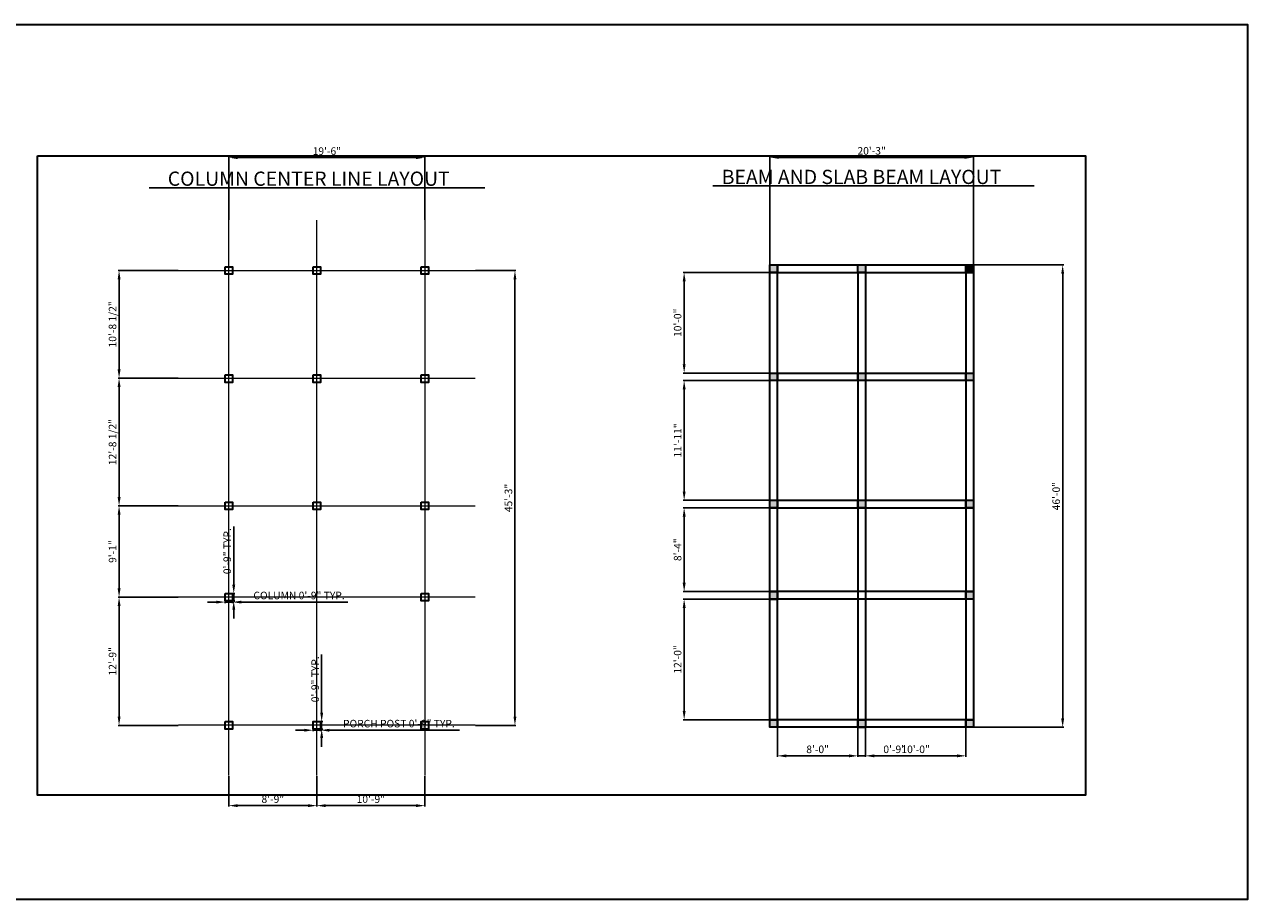
# Model space of a CAD drawing. Units: inches. Extents: x 1956 to 4770, y 1551 to 2596.
# Tile 10 of 10: x 3310 to 4770, y 1551 to 2596. Entities that reach past the tile are written whole.
import ezdxf

# ---------------------------------------------------------------- set-up
doc = ezdxf.new("R2010")
doc.units = ezdxf.units.IN
doc.linetypes.add('ACAD_ISO02W100', pattern=[15, 12, -3])
for name, color, linetype, lineweight in [('A-ANNO-DIMS', 2, 'Continuous', 18), ('A-ANNO-TITL', 6, 'Continuous', 25), ('A-ANNO-TTLB', 7, 'Continuous', 35), ('S-BEAM', 7, 'Continuous', 35), ('S-COLS', 5, 'Continuous', 35), ('S-COLS-HIDN', 5, 'ACAD_ISO02W100', 18), ('S-COLS-PATT', 1, 'Continuous', 13), ('S-GRID', 1, 'Continuous', 13)]:
    doc.layers.add(name, color=color, linetype=linetype, lineweight=lineweight)
doc.styles.get("Standard").update_dxf_attribs({"font": 'arial.ttf'})
doc.dimstyles.new('ISO-25', dxfattribs={"dimtxt": 9, "dimasz": 10.5, "dimexe": 1.25, "dimexo": 0.625, "dimgap": 2, "dimtad": 1, "dimdec": 1, "dimlunit": 4, "dimtxsty": 'Standard', "dimcen": 2.5, "dimadec": 0, "dimazin": 0, "dimtfac": 1, "dimtdec": 1, "dimtmove": 0, "dimatfit": 3, "dimfxl": 1, "dimarcsym": 0})

# ---------------------------------------------------------------- blocks, each defined once
blk = doc.blocks.new('COL-9X9-PLAN')
blk.add_lwpolyline([(0, 9), (9, 9), (9, 0), (0, 0)], close=True)
blk = doc.blocks.new('COL-PORCH-9X9')
blk.add_line((0, 0), (9, 0))
blk.add_lwpolyline([(0, 0), (0, 9), (9, 9), (9, 0)])
blk = doc.blocks.new('*D23')
at = {"layer": 'A-ANNO-DIMS', "color": 0, "lineweight": -2, "transparency": 16777216}
for p, q in [((3538.6, 1906.6), (3528.1, 1906.6)), ((3549.1, 1907.3), (3549.1, 1905.3)), ((3549.1, 1906.6), (3558.1, 1906.6)), ((3558.1, 1907.3), (3558.1, 1905.3)), ((3568.6, 1906.6), (3695.8, 1906.6))]:
    blk.add_line(p, q, dxfattribs=at)
at = {"layer": 'A-ANNO-DIMS', "color": 0, "transparency": 16777216}
for points in [[(3538.6, 1908.3), (3538.6, 1904.8), (3549.1, 1906.6)], [(3568.6, 1908.3), (3568.6, 1904.8), (3558.1, 1906.6)]]:
    blk.add_solid(points, dxfattribs=at)
at = {"layer": 'Defpoints', "color": 0, "transparency": 16777216}
for p in [(3549.1, 1907.9), (3558.1, 1907.9), (3558.1, 1906.6)]:
    blk.add_point(p, dxfattribs=at)
at = {"layer": 'A-ANNO-DIMS', "color": 0, "transparency": 16777216, "insert": (3637.4, 1913.3), "char_height": 9, "attachment_point": 5}
blk.add_mtext('COLUMN 0\'-9" TYP.', dxfattribs=at)
blk = doc.blocks.new('*D24')
at = {"layer": 'A-ANNO-DIMS', "color": 0, "lineweight": -2, "transparency": 16777216}
for p, q in [((3559.4, 1927.4), (3559.4, 1996.8)), ((3558.7, 1916.9), (3560.7, 1916.9)), ((3559.4, 1907.9), (3559.4, 1916.9)), ((3558.7, 1907.9), (3560.7, 1907.9)), ((3559.4, 1897.4), (3559.4, 1886.9))]:
    blk.add_line(p, q, dxfattribs=at)
at = {"layer": 'A-ANNO-DIMS', "color": 0, "transparency": 16777216}
for points in [[(3557.7, 1927.4), (3561.2, 1927.4), (3559.4, 1916.9)], [(3557.7, 1897.4), (3561.2, 1897.4), (3559.4, 1907.9)]]:
    blk.add_solid(points, dxfattribs=at)
at = {"layer": 'Defpoints', "color": 0, "transparency": 16777216}
for p in [(3558.1, 1916.9), (3559.4, 1916.9), (3558.1, 1907.9)]:
    blk.add_point(p, dxfattribs=at)
at = {"layer": 'A-ANNO-DIMS', "color": 0, "transparency": 16777216, "insert": (3552.8, 1967.4), "char_height": 9, "attachment_point": 5, "rotation": 90}
blk.add_mtext('0\'-9" TYP.', dxfattribs=at)
blk = doc.blocks.new('*D25')
at = {"layer": 'A-ANNO-DIMS', "color": 0, "lineweight": -2, "transparency": 16777216}
for p, q in [((3643.6, 1753.6), (3633.1, 1753.6)), ((3654.1, 1754.3), (3654.1, 1752.3)), ((3654.1, 1753.6), (3663.1, 1753.6)), ((3663.1, 1754.3), (3663.1, 1752.3)), ((3673.6, 1753.6), (3829.1, 1753.6))]:
    blk.add_line(p, q, dxfattribs=at)
at = {"layer": 'A-ANNO-DIMS', "color": 0, "transparency": 16777216}
for points in [[(3643.6, 1755.3), (3643.6, 1751.8), (3654.1, 1753.6)], [(3673.6, 1755.3), (3673.6, 1751.8), (3663.1, 1753.6)]]:
    blk.add_solid(points, dxfattribs=at)
at = {"layer": 'Defpoints', "color": 0, "transparency": 16777216}
for p in [(3654.1, 1754.9), (3663.1, 1754.9), (3663.1, 1753.6)]:
    blk.add_point(p, dxfattribs=at)
at = {"layer": 'A-ANNO-DIMS', "color": 0, "transparency": 16777216, "insert": (3756.6, 1760.3), "char_height": 9, "attachment_point": 5}
blk.add_mtext('PORCH POST 0\'-9" TYP.', dxfattribs=at)
blk = doc.blocks.new('*D26')
at = {"layer": 'A-ANNO-DIMS', "color": 0, "lineweight": -2, "transparency": 16777216}
for p, q in [((3664.4, 1774.4), (3664.4, 1843.8)), ((3663.7, 1763.9), (3665.7, 1763.9)), ((3663.7, 1754.9), (3665.7, 1754.9)), ((3664.4, 1754.9), (3664.4, 1763.9)), ((3664.4, 1744.4), (3664.4, 1733.9))]:
    blk.add_line(p, q, dxfattribs=at)
at = {"layer": 'A-ANNO-DIMS', "color": 0, "transparency": 16777216}
for points in [[(3662.7, 1774.4), (3666.2, 1774.4), (3664.4, 1763.9)], [(3662.7, 1744.4), (3666.2, 1744.4), (3664.4, 1754.9)]]:
    blk.add_solid(points, dxfattribs=at)
at = {"layer": 'Defpoints', "color": 0, "transparency": 16777216}
for p in [(3663.1, 1763.9), (3663.1, 1754.9), (3664.4, 1763.9)]:
    blk.add_point(p, dxfattribs=at)
at = {"layer": 'A-ANNO-DIMS', "color": 0, "transparency": 16777216, "insert": (3657.8, 1814.4), "char_height": 9, "attachment_point": 5, "rotation": 90}
blk.add_mtext('0\'-9" TYP.', dxfattribs=at)
blk = doc.blocks.new('*D87')
at = {"layer": 'A-ANNO-DIMS', "color": 0, "lineweight": -2, "transparency": 16777216}
for p, q in [((3553.6, 1698.8), (3553.6, 1662.3)), ((3658.6, 1698.8), (3658.6, 1662.3)), ((3564.1, 1663.5), (3648.1, 1663.5))]:
    blk.add_line(p, q, dxfattribs=at)
at = {"layer": 'A-ANNO-DIMS', "color": 0, "transparency": 16777216}
for points in [[(3564.1, 1665.3), (3564.1, 1661.8), (3553.6, 1663.5)], [(3648.1, 1665.3), (3648.1, 1661.8), (3658.6, 1663.5)]]:
    blk.add_solid(points, dxfattribs=at)
at = {"layer": 'Defpoints', "color": 0, "transparency": 16777216}
for p in [(3553.6, 1699.4), (3658.6, 1699.4), (3658.6, 1663.5)]:
    blk.add_point(p, dxfattribs=at)
at = {"layer": 'A-ANNO-DIMS', "color": 0, "transparency": 16777216, "insert": (3606.1, 1670.1), "char_height": 9, "attachment_point": 5}
blk.add_mtext('8\'-9"', dxfattribs=at)
blk = doc.blocks.new('*D88')
at = {"layer": 'A-ANNO-DIMS', "color": 0, "lineweight": -2, "transparency": 16777216}
for p, q in [((3658.6, 1698.8), (3658.6, 1662.3)), ((3787.6, 1698.8), (3787.6, 1662.3)), ((3669.1, 1663.5), (3777.1, 1663.5))]:
    blk.add_line(p, q, dxfattribs=at)
at = {"layer": 'A-ANNO-DIMS', "color": 0, "transparency": 16777216}
for points in [[(3669.1, 1665.3), (3669.1, 1661.8), (3658.6, 1663.5)], [(3777.1, 1665.3), (3777.1, 1661.8), (3787.6, 1663.5)]]:
    blk.add_solid(points, dxfattribs=at)
at = {"layer": 'Defpoints', "color": 0, "transparency": 16777216}
for p in [(3658.6, 1699.4), (3787.6, 1699.4), (3787.6, 1663.5)]:
    blk.add_point(p, dxfattribs=at)
at = {"layer": 'A-ANNO-DIMS', "color": 0, "transparency": 16777216, "insert": (3723.1, 1670.1), "char_height": 9, "attachment_point": 5}
blk.add_mtext('10\'-9"', dxfattribs=at)
blk = doc.blocks.new('*D89')
at = {"layer": 'A-ANNO-DIMS', "color": 0, "lineweight": -2, "transparency": 16777216}
for p, q in [((3492.9, 1912.4), (3421.3, 1912.4)), ((3422.5, 1769.9), (3422.5, 1901.9)), ((3492.9, 1759.4), (3421.3, 1759.4))]:
    blk.add_line(p, q, dxfattribs=at)
at = {"layer": 'A-ANNO-DIMS', "color": 0, "transparency": 16777216}
for points in [[(3420.8, 1901.9), (3424.3, 1901.9), (3422.5, 1912.4)], [(3420.8, 1769.9), (3424.3, 1769.9), (3422.5, 1759.4)]]:
    blk.add_solid(points, dxfattribs=at)
at = {"layer": 'Defpoints', "color": 0, "transparency": 16777216}
for p in [(3422.5, 1912.4), (3493.6, 1912.4), (3493.6, 1759.4)]:
    blk.add_point(p, dxfattribs=at)
at = {"layer": 'A-ANNO-DIMS', "color": 0, "transparency": 16777216, "insert": (3415.9, 1835.9), "char_height": 9, "attachment_point": 5, "rotation": 90}
blk.add_mtext('12\'-9"', dxfattribs=at)
blk = doc.blocks.new('*D90')
at = {"layer": 'A-ANNO-DIMS', "color": 0, "lineweight": -2, "transparency": 16777216}
for p, q in [((3492.9, 2021.4), (3421.3, 2021.4)), ((3422.5, 1922.9), (3422.5, 2010.9)), ((3492.9, 1912.4), (3421.3, 1912.4))]:
    blk.add_line(p, q, dxfattribs=at)
at = {"layer": 'A-ANNO-DIMS', "color": 0, "transparency": 16777216}
for points in [[(3420.8, 2010.9), (3424.3, 2010.9), (3422.5, 2021.4)], [(3420.8, 1922.9), (3424.3, 1922.9), (3422.5, 1912.4)]]:
    blk.add_solid(points, dxfattribs=at)
at = {"layer": 'Defpoints', "color": 0, "transparency": 16777216}
for p in [(3422.5, 2021.4), (3493.6, 2021.4), (3493.6, 1912.4)]:
    blk.add_point(p, dxfattribs=at)
at = {"layer": 'A-ANNO-DIMS', "color": 0, "transparency": 16777216, "insert": (3415.9, 1966.9), "char_height": 9, "attachment_point": 5, "rotation": 90}
blk.add_mtext('9\'-1"', dxfattribs=at)
blk = doc.blocks.new('*D91')
at = {"layer": 'A-ANNO-DIMS', "color": 0, "lineweight": -2, "transparency": 16777216}
for p, q in [((3492.9, 2173.9), (3421.3, 2173.9)), ((3422.5, 2031.9), (3422.5, 2163.4)), ((3492.9, 2021.4), (3421.3, 2021.4))]:
    blk.add_line(p, q, dxfattribs=at)
at = {"layer": 'A-ANNO-DIMS', "color": 0, "transparency": 16777216}
for points in [[(3420.8, 2163.4), (3424.3, 2163.4), (3422.5, 2173.9)], [(3420.8, 2031.9), (3424.3, 2031.9), (3422.5, 2021.4)]]:
    blk.add_solid(points, dxfattribs=at)
at = {"layer": 'Defpoints', "color": 0, "transparency": 16777216}
for p in [(3422.5, 2173.9), (3493.6, 2173.9), (3493.6, 2021.4)]:
    blk.add_point(p, dxfattribs=at)
at = {"layer": 'A-ANNO-DIMS', "color": 0, "transparency": 16777216, "insert": (3415.9, 2097.7), "char_height": 9, "attachment_point": 5, "rotation": 90}
blk.add_mtext('12\'-8 1/2"', dxfattribs=at)
blk = doc.blocks.new('*D92')
at = {"layer": 'A-ANNO-DIMS', "color": 0, "lineweight": -2, "transparency": 16777216}
for p, q in [((3492.9, 2302.4), (3421.3, 2302.4)), ((3422.5, 2184.4), (3422.5, 2291.9)), ((3492.9, 2173.9), (3421.3, 2173.9))]:
    blk.add_line(p, q, dxfattribs=at)
at = {"layer": 'A-ANNO-DIMS', "color": 0, "transparency": 16777216}
for points in [[(3420.8, 2291.9), (3424.3, 2291.9), (3422.5, 2302.4)], [(3420.8, 2184.4), (3424.3, 2184.4), (3422.5, 2173.9)]]:
    blk.add_solid(points, dxfattribs=at)
at = {"layer": 'Defpoints', "color": 0, "transparency": 16777216}
for p in [(3422.5, 2302.4), (3493.6, 2302.4), (3493.6, 2173.9)]:
    blk.add_point(p, dxfattribs=at)
at = {"layer": 'A-ANNO-DIMS', "color": 0, "transparency": 16777216, "insert": (3415.9, 2238.2), "char_height": 9, "attachment_point": 5, "rotation": 90}
blk.add_mtext('10\'-8 1/2"', dxfattribs=at)
blk = doc.blocks.new('*D93')
at = {"layer": 'A-ANNO-DIMS', "color": 0, "lineweight": -2, "transparency": 16777216}
for p, q in [((3553.6, 2363.1), (3553.6, 2438.5)), ((3564.1, 2437.3), (3777.1, 2437.3)), ((3787.6, 2363.1), (3787.6, 2438.5))]:
    blk.add_line(p, q, dxfattribs=at)
at = {"layer": 'A-ANNO-DIMS', "color": 0, "transparency": 16777216}
for points in [[(3564.1, 2439), (3564.1, 2435.5), (3553.6, 2437.3)], [(3777.1, 2439), (3777.1, 2435.5), (3787.6, 2437.3)]]:
    blk.add_solid(points, dxfattribs=at)
at = {"layer": 'Defpoints', "color": 0, "transparency": 16777216}
for p in [(3787.6, 2437.3), (3553.6, 2362.4), (3787.6, 2362.4)]:
    blk.add_point(p, dxfattribs=at)
at = {"layer": 'A-ANNO-DIMS', "color": 0, "transparency": 16777216, "insert": (3670.6, 2443.9), "char_height": 9, "attachment_point": 5}
blk.add_mtext('19\'-6"', dxfattribs=at)
blk = doc.blocks.new('*D94')
at = {"layer": 'A-ANNO-DIMS', "color": 0, "lineweight": -2, "transparency": 16777216}
for p, q in [((3848.2, 2302.4), (3896.4, 2302.4)), ((3895.2, 1769.9), (3895.2, 2291.9)), ((3848.2, 1759.4), (3896.4, 1759.4))]:
    blk.add_line(p, q, dxfattribs=at)
at = {"layer": 'A-ANNO-DIMS', "color": 0, "transparency": 16777216}
for points in [[(3893.4, 2291.9), (3896.9, 2291.9), (3895.2, 2302.4)], [(3893.4, 1769.9), (3896.9, 1769.9), (3895.2, 1759.4)]]:
    blk.add_solid(points, dxfattribs=at)
at = {"layer": 'Defpoints', "color": 0, "transparency": 16777216}
for p in [(3847.6, 2302.4), (3895.2, 2302.4), (3847.6, 1759.4)]:
    blk.add_point(p, dxfattribs=at)
at = {"layer": 'A-ANNO-DIMS', "color": 0, "transparency": 16777216, "insert": (3888.6, 2030.9), "char_height": 9, "attachment_point": 5, "rotation": 90}
blk.add_mtext('45\'-3"', dxfattribs=at)
blk = doc.blocks.new('*D95')
at = {"layer": 'A-ANNO-DIMS', "color": 0, "lineweight": -2, "transparency": 16777216}
for p, q in [((4199.6, 2309.7), (4199.6, 2438.8)), ((4442.6, 2309.7), (4442.6, 2438.8)), ((4210.1, 2437.6), (4432.1, 2437.6))]:
    blk.add_line(p, q, dxfattribs=at)
at = {"layer": 'A-ANNO-DIMS', "color": 0, "transparency": 16777216}
for points in [[(4210.1, 2439.3), (4210.1, 2435.8), (4199.6, 2437.6)], [(4432.1, 2439.3), (4432.1, 2435.8), (4442.6, 2437.6)]]:
    blk.add_solid(points, dxfattribs=at)
at = {"layer": 'Defpoints', "color": 0, "transparency": 16777216}
for p in [(4442.6, 2437.6), (4199.6, 2309.1), (4442.6, 2309.1)]:
    blk.add_point(p, dxfattribs=at)
at = {"layer": 'A-ANNO-DIMS', "color": 0, "transparency": 16777216, "insert": (4321.1, 2444.2), "char_height": 9, "attachment_point": 5}
blk.add_mtext('20\'-3"', dxfattribs=at)
blk = doc.blocks.new('*D96')
at = {"layer": 'A-ANNO-DIMS', "color": 0, "lineweight": -2, "transparency": 16777216}
for p, q in [((4443.2, 2309.1), (4550.4, 2309.1)), ((4549.2, 1767.6), (4549.2, 2298.6)), ((4443.2, 1757.1), (4550.4, 1757.1))]:
    blk.add_line(p, q, dxfattribs=at)
at = {"layer": 'A-ANNO-DIMS', "color": 0, "transparency": 16777216}
for points in [[(4547.4, 2298.6), (4550.9, 2298.6), (4549.2, 2309.1)], [(4547.4, 1767.6), (4550.9, 1767.6), (4549.2, 1757.1)]]:
    blk.add_solid(points, dxfattribs=at)
at = {"layer": 'Defpoints', "color": 0, "transparency": 16777216}
for p in [(4442.6, 2309.1), (4549.2, 2309.1), (4442.6, 1757.1)]:
    blk.add_point(p, dxfattribs=at)
at = {"layer": 'A-ANNO-DIMS', "color": 0, "transparency": 16777216, "insert": (4542.6, 2033.1), "char_height": 9, "attachment_point": 5, "rotation": 90}
blk.add_mtext('46\'-0"', dxfattribs=at)
blk = doc.blocks.new('*D97')
at = {"layer": 'A-ANNO-DIMS', "color": 0, "lineweight": -2, "transparency": 16777216}
for p, q in [((4208.6, 1765.5), (4208.6, 1721.7)), ((4304.6, 1765.5), (4304.6, 1721.7)), ((4219.1, 1723), (4294.1, 1723))]:
    blk.add_line(p, q, dxfattribs=at)
at = {"layer": 'A-ANNO-DIMS', "color": 0, "transparency": 16777216}
for points in [[(4219.1, 1724.7), (4219.1, 1721.2), (4208.6, 1723)], [(4294.1, 1724.7), (4294.1, 1721.2), (4304.6, 1723)]]:
    blk.add_solid(points, dxfattribs=at)
at = {"layer": 'Defpoints', "color": 0, "transparency": 16777216}
for p in [(4208.6, 1766.1), (4304.6, 1766.1), (4304.6, 1723)]:
    blk.add_point(p, dxfattribs=at)
at = {"layer": 'A-ANNO-DIMS', "color": 0, "transparency": 16777216, "insert": (4256.6, 1729.6), "char_height": 9, "attachment_point": 5}
blk.add_mtext('8\'-0"', dxfattribs=at)
blk = doc.blocks.new('*D98')
at = {"layer": 'A-ANNO-DIMS', "color": 0, "lineweight": -2, "transparency": 16777216}
for p, q in [((4313.6, 1765.5), (4313.6, 1721.7)), ((4433.6, 1765.5), (4433.6, 1721.7)), ((4324.1, 1723), (4423.1, 1723))]:
    blk.add_line(p, q, dxfattribs=at)
at = {"layer": 'A-ANNO-DIMS', "color": 0, "transparency": 16777216}
for points in [[(4324.1, 1724.7), (4324.1, 1721.2), (4313.6, 1723)], [(4423.1, 1724.7), (4423.1, 1721.2), (4433.6, 1723)]]:
    blk.add_solid(points, dxfattribs=at)
at = {"layer": 'Defpoints', "color": 0, "transparency": 16777216}
for p in [(4313.6, 1766.1), (4433.6, 1766.1), (4433.6, 1723)]:
    blk.add_point(p, dxfattribs=at)
at = {"layer": 'A-ANNO-DIMS', "color": 0, "transparency": 16777216, "insert": (4373.6, 1729.6), "char_height": 9, "attachment_point": 5}
blk.add_mtext('10\'-0"', dxfattribs=at)
blk = doc.blocks.new('*D99')
at = {"layer": 'A-ANNO-DIMS', "color": 0, "lineweight": -2, "transparency": 16777216}
for p, q in [((4304.6, 1756.5), (4304.6, 1721.7)), ((4313.6, 1756.5), (4313.6, 1721.7)), ((4294.1, 1723), (4283.6, 1723)), ((4304.6, 1723), (4313.6, 1723)), ((4324.1, 1723), (4362.5, 1723))]:
    blk.add_line(p, q, dxfattribs=at)
at = {"layer": 'A-ANNO-DIMS', "color": 0, "transparency": 16777216}
for points in [[(4294.1, 1724.7), (4294.1, 1721.2), (4304.6, 1723)], [(4324.1, 1724.7), (4324.1, 1721.2), (4313.6, 1723)]]:
    blk.add_solid(points, dxfattribs=at)
at = {"layer": 'Defpoints', "color": 0, "transparency": 16777216}
for p in [(4304.6, 1757.1), (4313.6, 1757.1), (4313.6, 1723)]:
    blk.add_point(p, dxfattribs=at)
at = {"layer": 'A-ANNO-DIMS', "color": 0, "transparency": 16777216, "insert": (4348.6, 1729.6), "char_height": 9, "attachment_point": 5}
blk.add_mtext('0\'-9"', dxfattribs=at)
blk = doc.blocks.new('*D100')
at = {"layer": 'A-ANNO-DIMS', "color": 0, "lineweight": -2, "transparency": 16777216}
for p, q in [((4199, 1910.1), (4096, 1910.1)), ((4097.2, 1776.6), (4097.2, 1899.6)), ((4199, 1766.1), (4096, 1766.1))]:
    blk.add_line(p, q, dxfattribs=at)
at = {"layer": 'A-ANNO-DIMS', "color": 0, "transparency": 16777216}
for points in [[(4095.5, 1899.6), (4099, 1899.6), (4097.2, 1910.1)], [(4095.5, 1776.6), (4099, 1776.6), (4097.2, 1766.1)]]:
    blk.add_solid(points, dxfattribs=at)
at = {"layer": 'Defpoints', "color": 0, "transparency": 16777216}
for p in [(4097.2, 1910.1), (4199.6, 1910.1), (4199.6, 1766.1)]:
    blk.add_point(p, dxfattribs=at)
at = {"layer": 'A-ANNO-DIMS', "color": 0, "transparency": 16777216, "insert": (4090.6, 1838.1), "char_height": 9, "attachment_point": 5, "rotation": 90}
blk.add_mtext('12\'-0"', dxfattribs=at)
blk = doc.blocks.new('*D101')
at = {"layer": 'A-ANNO-DIMS', "color": 0, "lineweight": -2, "transparency": 16777216}
for p, q in [((4199, 2019.1), (4096, 2019.1)), ((4097.2, 1929.6), (4097.2, 2008.6)), ((4199, 1919.1), (4096, 1919.1))]:
    blk.add_line(p, q, dxfattribs=at)
at = {"layer": 'A-ANNO-DIMS', "color": 0, "transparency": 16777216}
for points in [[(4095.5, 2008.6), (4099, 2008.6), (4097.2, 2019.1)], [(4095.5, 1929.6), (4099, 1929.6), (4097.2, 1919.1)]]:
    blk.add_solid(points, dxfattribs=at)
at = {"layer": 'Defpoints', "color": 0, "transparency": 16777216}
for p in [(4097.2, 2019.1), (4199.6, 2019.1), (4199.6, 1919.1)]:
    blk.add_point(p, dxfattribs=at)
at = {"layer": 'A-ANNO-DIMS', "color": 0, "transparency": 16777216, "insert": (4090.6, 1969.1), "char_height": 9, "attachment_point": 5, "rotation": 90}
blk.add_mtext('8\'-4"', dxfattribs=at)
blk = doc.blocks.new('*D102')
at = {"layer": 'A-ANNO-DIMS', "color": 0, "lineweight": -2, "transparency": 16777216}
for p, q in [((4199, 2171.1), (4096, 2171.1)), ((4097.2, 2038.6), (4097.2, 2160.6)), ((4199, 2028.1), (4096, 2028.1))]:
    blk.add_line(p, q, dxfattribs=at)
at = {"layer": 'A-ANNO-DIMS', "color": 0, "transparency": 16777216}
for points in [[(4095.5, 2160.6), (4099, 2160.6), (4097.2, 2171.1)], [(4095.5, 2038.6), (4099, 2038.6), (4097.2, 2028.1)]]:
    blk.add_solid(points, dxfattribs=at)
at = {"layer": 'Defpoints', "color": 0, "transparency": 16777216}
for p in [(4097.2, 2171.1), (4199.6, 2171.1), (4199.6, 2028.1)]:
    blk.add_point(p, dxfattribs=at)
at = {"layer": 'A-ANNO-DIMS', "color": 0, "transparency": 16777216, "insert": (4090.7, 2099.6), "char_height": 9, "attachment_point": 5, "rotation": 90}
blk.add_mtext('11\'-11"', dxfattribs=at)
blk = doc.blocks.new('*D103')
at = {"layer": 'A-ANNO-DIMS', "color": 0, "lineweight": -2, "transparency": 16777216}
for p, q in [((4199, 2300.1), (4096, 2300.1)), ((4097.2, 2190.6), (4097.2, 2289.6)), ((4199, 2180.1), (4096, 2180.1))]:
    blk.add_line(p, q, dxfattribs=at)
at = {"layer": 'A-ANNO-DIMS', "color": 0, "transparency": 16777216}
for points in [[(4095.5, 2289.6), (4099, 2289.6), (4097.2, 2300.1)], [(4095.5, 2190.6), (4099, 2190.6), (4097.2, 2180.1)]]:
    blk.add_solid(points, dxfattribs=at)
at = {"layer": 'Defpoints', "color": 0, "transparency": 16777216}
for p in [(4097.2, 2300.1), (4199.6, 2300.1), (4199.6, 2180.1)]:
    blk.add_point(p, dxfattribs=at)
at = {"layer": 'A-ANNO-DIMS', "color": 0, "transparency": 16777216, "insert": (4090.6, 2240.1), "char_height": 9, "attachment_point": 5, "rotation": 90}
blk.add_mtext('10\'-0"', dxfattribs=at)

msp = doc.modelspace()

# ---------------------------------------------------------------- hatches: boundary and pattern name
at = {"layer": 'S-COLS-PATT'}
h = msp.add_hatch(color=256, dxfattribs=at)
h.dxf.hatch_style = 1
h.paths.add_polyline_path([(4313.62, 2309.09), (4304.62, 2309.09), (4304.62, 2300.09), (4313.62, 2300.09)])
h.paths.add_polyline_path([(4208.62, 2309.09), (4199.62, 2309.09), (4199.62, 2300.09), (4208.62, 2300.09)])
h.paths.add_polyline_path([(4208.62, 2180.09), (4199.62, 2180.09), (4199.62, 2171.59), (4208.62, 2171.59)])
h.paths.add_polyline_path([(4313.62, 2180.09), (4304.62, 2180.09), (4304.62, 2171.59), (4313.62, 2171.59)])
h.paths.add_polyline_path([(4442.62, 2180.09), (4433.62, 2180.09), (4433.62, 2171.59), (4442.62, 2171.59)])
h.paths.add_polyline_path([(4208.62, 2028.09), (4199.62, 2028.09), (4199.62, 2019.09), (4208.62, 2019.09)])
h.paths.add_polyline_path([(4313.62, 2028.09), (4304.62, 2028.09), (4304.62, 2019.09), (4313.62, 2019.09)])
h.paths.add_polyline_path([(4442.62, 2028.09), (4433.62, 2028.09), (4433.62, 2019.09), (4442.62, 2019.09)])
h.paths.add_polyline_path([(4442.62, 1919.09), (4433.62, 1919.09), (4433.62, 1910.09), (4442.62, 1910.09)])
h.paths.add_polyline_path([(4208.62, 1919.09), (4199.62, 1919.09), (4199.62, 1910.09), (4208.62, 1910.09)])
h.paths.add_polyline_path([(4208.62, 1766.09), (4199.62, 1766.09), (4199.62, 1761.59), (4208.62, 1761.59)])
h.paths.add_polyline_path([(4208.62, 1761.59), (4199.62, 1761.59), (4199.62, 1757.09), (4208.62, 1757.09)])
h.paths.add_polyline_path([(4313.62, 1766.09), (4304.62, 1766.09), (4304.62, 1761.59), (4313.62, 1761.59)])
h.paths.add_polyline_path([(4313.62, 1761.59), (4304.62, 1761.59), (4304.62, 1757.09), (4313.62, 1757.09)])
h.paths.add_polyline_path([(4442.62, 1766.09), (4433.62, 1766.09), (4433.62, 1761.59), (4442.62, 1761.59)])
h.paths.add_polyline_path([(4442.62, 1761.59), (4433.62, 1761.59), (4433.62, 1757.09), (4442.62, 1757.09)])
h = msp.add_hatch(color=256, dxfattribs=at)
h.dxf.hatch_style = 1
h.paths.add_polyline_path([(4442.62, 2309.09), (4433.62, 2309.09), (4433.62, 2300.09), (4442.62, 2300.09)])

# ---------------------------------------------------------------- linework, layer by layer
at = {"layer": 'A-ANNO-TITL'}
for p, q in [((3458.46, 2401.36), (3859.27, 2401.36)), ((4131.34, 2403.5), (4515.05, 2403.5))]:
    msp.add_line(p, q, dxfattribs=at)
at = {"layer": 'A-ANNO-TTLB'}
for points in [[(1955.79, 2596.29), (4769.89, 2596.29), (4769.89, 1551.4), (1955.79, 1551.4)], [(3325.16, 2439.33), (4576.44, 2439.33), (4576.44, 1676.04), (3325.16, 1676.04)]]:
    msp.add_lwpolyline(points, close=True, dxfattribs=at)
at = {"layer": 'S-BEAM'}
for p, q in [((4199.62, 2309.09), (4442.62, 2309.09)), ((4199.62, 1757.09), (4199.62, 2309.09)), ((4208.62, 1757.09), (4208.62, 2309.09)), ((4433.62, 2309.09), (4433.62, 1757.09)), ((4442.62, 2309.09), (4442.62, 1757.09)), ((4199.62, 2300.09), (4442.62, 2300.09)), ((4304.62, 2300.09), (4304.62, 1757.09)), ((4313.62, 2300.09), (4313.62, 1757.09)), ((4199.62, 2180.09), (4442.62, 2180.09)), ((4199.62, 2171.59), (4442.62, 2171.59)), ((4199.62, 2028.09), (4442.62, 2028.09)), ((4199.62, 2019.09), (4442.62, 2019.09)), ((4442.62, 1919.09), (4199.62, 1919.09)), ((4442.62, 1910.09), (4199.62, 1910.09)), ((4442.62, 1766.09), (4199.62, 1766.09)), ((4442.62, 1757.09), (4199.62, 1757.09))]:
    msp.add_line(p, q, dxfattribs=at)
at = {"layer": 'S-COLS'}
for p, q in [((3654.06, 2306.95), (3663.06, 2306.95)), ((3783.06, 2306.95), (3792.06, 2306.95)), ((3549.06, 1907.95), (3558.06, 1907.95)), ((4199.62, 1910.09), (4208.62, 1910.09))]:
    msp.add_line(p, q, dxfattribs=at)
for points in [[(4433.62, 2309.09), (4442.62, 2309.09), (4442.62, 2300.09), (4433.62, 2300.09)], [(4433.62, 2309.09), (4442.62, 2309.09), (4442.62, 2300.09), (4433.62, 2300.09)], [(3783.06, 2306.95), (3792.06, 2306.95), (3792.06, 2297.95), (3783.06, 2297.95)], [(3783.06, 2306.95), (3792.06, 2306.95), (3792.06, 2297.95), (3783.06, 2297.95)], [(3654.06, 1763.95), (3663.06, 1763.95), (3663.06, 1754.95), (3654.06, 1754.95)], [(4304.62, 1766.09), (4313.62, 1766.09), (4313.62, 1757.09), (4304.62, 1757.09)]]:
    msp.add_lwpolyline(points, close=True, dxfattribs=at)
for points in [[(3783.06, 1754.95), (3783.06, 1763.95), (3792.06, 1763.95), (3792.06, 1754.95)], [(4433.62, 1757.09), (4433.62, 1766.09), (4442.62, 1766.09), (4442.62, 1757.09)]]:
    msp.add_lwpolyline(points, dxfattribs=at)
at = {"layer": 'S-COLS-HIDN'}
for p, q in [((3654.06, 1754.95), (3654.06, 1763.95)), ((4304.62, 1757.09), (4304.62, 1766.09))]:
    msp.add_line(p, q, dxfattribs=at)
at = {"layer": 'S-GRID'}
for p, q in [((3553.56, 1699.45), (3553.56, 2362.45)), ((3658.56, 1699.45), (3658.56, 2362.45)), ((3787.56, 2362.45), (3787.56, 1699.45)), ((3493.56, 2302.45), (3847.56, 2302.45)), ((3493.56, 2173.95), (3792.06, 2173.95)), ((3783.06, 2173.95), (3847.56, 2173.95)), ((3493.56, 2021.45), (3847.5, 2021.45)), ((3847.56, 1912.45), (3493.56, 1912.45)), ((3847.56, 1759.45), (3493.56, 1759.45))]:
    msp.add_line(p, q, dxfattribs=at)

# ---------------------------------------------------------------- block references
at = {"layer": 'S-COLS'}
for name, p in [('COL-9X9-PLAN', (4199.62, 2300.09)), ('COL-9X9-PLAN', (4304.62, 2300.09)), ('COL-9X9-PLAN', (4433.62, 2300.09)), ('COL-9X9-PLAN', (3549.06, 2297.95)), ('COL-9X9-PLAN', (3654.06, 2297.95)), ('COL-9X9-PLAN', (3783.06, 2297.95)), ('COL-9X9-PLAN', (3549.06, 2168.95)), ('COL-9X9-PLAN', (3654.06, 2168.95)), ('COL-9X9-PLAN', (3783.06, 2168.95)), ('COL-9X9-PLAN', (4199.62, 2171.09)), ('COL-9X9-PLAN', (4304.62, 2171.09)), ('COL-9X9-PLAN', (4433.62, 2171.09)), ('COL-9X9-PLAN', (3549.06, 2016.95)), ('COL-9X9-PLAN', (3654.06, 2016.95)), ('COL-9X9-PLAN', (3783.06, 2016.95)), ('COL-9X9-PLAN', (4199.62, 2019.09)), ('COL-9X9-PLAN', (4304.62, 2019.09)), ('COL-9X9-PLAN', (4433.62, 2019.09)), ('COL-9X9-PLAN', (3549.06, 1907.95)), ('COL-9X9-PLAN', (3783.06, 1907.95)), ('COL-9X9-PLAN', (4199.62, 1910.09)), ('COL-9X9-PLAN', (4433.62, 1910.09)), ('COL-9X9-PLAN', (3549.06, 1754.95)), ('COL-9X9-PLAN', (3654.06, 1754.95)), ('COL-PORCH-9X9', (3654.06, 1754.95)), ('COL-9X9-PLAN', (3783.06, 1754.95)), ('COL-9X9-PLAN', (4199.62, 1757.09)), ('COL-9X9-PLAN', (4304.62, 1757.09)), ('COL-PORCH-9X9', (4304.62, 1757.09)), ('COL-9X9-PLAN', (4433.62, 1757.09))]:
    msp.add_blockref(name, p, dxfattribs=at)

# ---------------------------------------------------------------- texts
at = {"layer": 'A-ANNO-TITL'}
for s, p in [('COLUMN CENTER LINE LAYOUT', (3480.65, 2403.62)), ('BEAM AND SLAB BEAM LAYOUT', (4142.09, 2405.75))]:
    msp.add_text(s, height=17, dxfattribs=at).set_placement(p)

# ---------------------------------------------------------------- dimensions: what is measured, and where the dimension line sits
at = {"layer": 'A-ANNO-DIMS'}
for base, p1, p2, picture, middle in [((3787.56, 2437.29), (3553.56, 2362.45), (3787.56, 2362.45), '*D93', (3670.56, 2443.89)), ((4442.62, 2437.6), (4199.62, 2309.09), (4442.62, 2309.09), '*D95', (4321.12, 2444.2)), ((4304.62, 1722.99), (4208.62, 1766.09), (4304.62, 1766.09), '*D97', (4256.62, 1729.58)), ((4313.62, 1722.99), (4304.62, 1757.09), (4313.62, 1757.09), '*D99', (4348.58, 1729.58)), ((4433.62, 1722.99), (4313.62, 1766.09), (4433.62, 1766.09), '*D98', (4373.62, 1729.58)), ((3658.56, 1663.52), (3553.56, 1699.45), (3658.56, 1699.45), '*D87', (3606.06, 1670.11)), ((3787.56, 1663.52), (3658.56, 1699.45), (3787.56, 1699.45), '*D88', (3723.06, 1670.11))]:
    dim = msp.add_linear_dim(base=base, p1=p1, p2=p2, dimstyle='ISO-25', override={"dimdec": 1, "dimlfac": 1, "dimrnd": 0, "dimzin": 1, "dimdsep": 46, "dimlunit": 4, "dimfrac": 2}, dxfattribs=at)
    dim.commit()
    dim.dimension.update_dxf_attribs({"geometry": picture, "text_midpoint": middle})
for base, p1, p2, picture, middle in [((4549.15, 2309.09), (4442.62, 1757.09), (4442.62, 2309.09), '*D96', (4542.56, 2033.09)), ((3422.53, 2302.45), (3493.56, 2173.95), (3493.56, 2302.45), '*D92', (3415.88, 2238.2)), ((3895.2, 2302.45), (3847.56, 1759.45), (3847.56, 2302.45), '*D94', (3888.6, 2030.95)), ((4097.24, 2300.09), (4199.62, 2180.09), (4199.62, 2300.09), '*D103', (4090.64, 2240.09)), ((3422.53, 2173.95), (3493.56, 2021.45), (3493.56, 2173.95), '*D91', (3415.88, 2097.7)), ((4097.24, 2171.09), (4199.62, 2028.09), (4199.62, 2171.09), '*D102', (4090.72, 2099.59)), ((3422.53, 2021.45), (3493.56, 1912.45), (3493.56, 2021.45), '*D90', (3415.94, 1966.95)), ((4097.24, 2019.09), (4199.62, 1919.09), (4199.62, 2019.09), '*D101', (4090.64, 1969.09)), ((3422.53, 1912.45), (3493.56, 1759.45), (3493.56, 1912.45), '*D89', (3415.94, 1835.95)), ((4097.24, 1910.09), (4199.62, 1766.09), (4199.62, 1910.09), '*D100', (4090.64, 1838.09))]:
    dim = msp.add_linear_dim(base=base, p1=p1, p2=p2, angle=90, dimstyle='ISO-25', override={"dimdec": 1, "dimlfac": 1, "dimrnd": 0, "dimzin": 1, "dimdsep": 46, "dimlunit": 4, "dimfrac": 2}, dxfattribs=at)
    dim.commit()
    dim.dimension.update_dxf_attribs({"geometry": picture, "text_midpoint": middle})
for base, p1, p2, picture, middle in [((3559.41, 1916.95), (3558.06, 1907.95), (3558.06, 1916.95), '*D24', (3552.81, 1967.38)), ((3664.41, 1763.95), (3663.06, 1754.95), (3663.06, 1763.95), '*D26', (3657.81, 1814.38))]:
    dim = msp.add_linear_dim(base=base, p1=p1, p2=p2, angle=90, text='<> TYP.', dimstyle='ISO-25', override={"dimdec": 1, "dimlfac": 1, "dimrnd": 0, "dimzin": 1, "dimdsep": 46, "dimlunit": 4, "dimfrac": 2}, dxfattribs=at)
    dim.commit()
    dim.dimension.update_dxf_attribs({"geometry": picture, "text_midpoint": middle})
for base, p1, p2, text, picture, middle in [((3558.06, 1906.6), (3549.06, 1907.95), (3558.06, 1907.95), 'COLUMN <> TYP.', '*D23', (3637.42, 1913.26)), ((3663.06, 1753.6), (3654.06, 1754.95), (3663.06, 1754.95), 'PORCH POST <> TYP.', '*D25', (3756.57, 1760.26))]:
    dim = msp.add_linear_dim(base=base, p1=p1, p2=p2, text=text, dimstyle='ISO-25', override={"dimdec": 1, "dimlfac": 1, "dimrnd": 0, "dimzin": 1, "dimdsep": 46, "dimlunit": 4, "dimfrac": 2}, dxfattribs=at)
    dim.commit()
    dim.dimension.update_dxf_attribs({"geometry": picture, "text_midpoint": middle})

doc.saveas('drawing.dxf')
